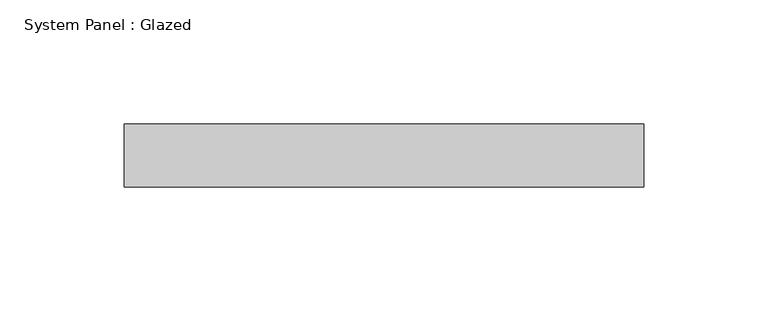
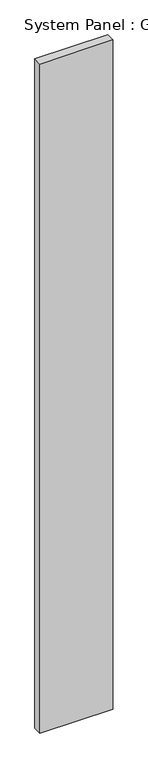
"""IFC4 building model written with IfcOpenShell, lengths in millimetres: plate geometry, System Panel : Glazed."""

from ifc_helpers import new_model, si_unit, origin, origin_with_axes, place, context, project, spatial, polyline, outline, extrude, source, transform, mapped, element, save


def system_panel_glazed_ab75977c(model_context):
    return source(origin(), model_context, "Body", "SweptSolid", [
        extrude(outline(polyline([(104.775, 19.05), (-104.775, 19.05), (-104.775, 44.45), (104.775, 44.45), (104.775, 19.05)])), origin_with_axes(), (0.0, 0.0, 1.0), 2038.35),
    ])


if __name__ == "__main__":
    model = new_model("IFC4")
    model_context = context("Model", 3, world=origin())
    ifc_project = project(units=[si_unit("LENGTHUNIT", "METRE", prefix="MILLI")], contexts=[model_context])
    site = spatial("IfcSite", under=ifc_project)
    building = spatial("IfcBuilding", under=site)
    placement = place(None, origin())
    system_panel_glazed_shape = system_panel_glazed_ab75977c(model_context)
    element("IfcPlate", 1, ObjectType="System Panel : Glazed", at=placement, inside=building, context=model_context, shape_type="MappedRepresentation", body=[
        mapped(system_panel_glazed_shape, transform((0.0, 0.0, 0.0), x_axis=(1.0, 0.0, 0.0), y_axis=(0.0, 1.0, 0.0), z_axis=(0.0, 0.0, 1.0))),
    ])
    save(model, "model.ifc")

# Revit data of these elements
# Type "System Panel : Glazed"
#   Construction Type Id = "GSP4R"
#   Analytic Construction = "1/8 in Pilkington single glazing"
#   Visual Light Transmittance = 0.9
#   Solar Heat Gain Coefficient = 0.86
#   Heat Transfer Coefficient (U) = 1.18115 BTU/(h·ft²·°F)
#   Define Thermal Properties by = 1
# Element 1 (IfcPlate, "System Panel : Glazed")
#   Materials on its faces: "Glass"
# Materials
#   "Glass": class "Glass", colour RGB 0 128 192, transparency 0.75, Description = "Soda Lime Glass", Cost = 0
